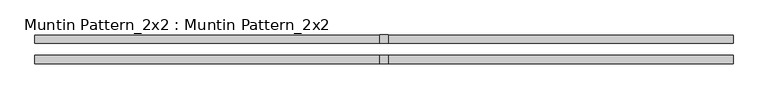
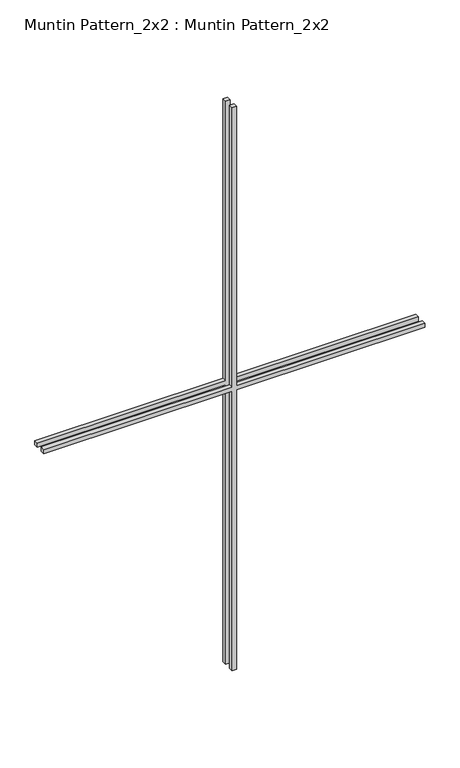
"""IFC4 building model written with IfcOpenShell, lengths in millimetres: proxy geometry, Muntin Pattern_2x2 : Muntin Pattern_2x2."""

from ifc_helpers import new_model, si_unit, frame, origin, place, context, project, spatial, polyline, outline, extrude, source, transform, mapped, element, save


def muntin_pattern_2x2_muntin_pattern_2x2_d03a1f3c(model_context):
    return source(origin(), model_context, "Body", "SweptSolid", [
        extrude(outline(polyline([(850.9, -6.35), (850.9, -541.3375), (838.2, -541.3375), (838.2, -6.35), (0.0, -6.35), (0.0, 6.35), (838.2, 6.35), (838.2, 541.3375), (850.9, 541.3375), (850.9, 6.35), (1689.1, 6.35), (1689.1, -6.35), (850.9, -6.35)])), frame((0.0, -22.225, 0.0), z_axis=(0.0, 1.0, 0.0), x_axis=(0.0, 0.0, 1.0)), (0.0, 0.0, 1.0), 12.7),
        extrude(outline(polyline([(850.9, -6.35), (850.9, -541.3375), (838.2, -541.3375), (838.2, -6.35), (0.0, -6.35), (0.0, 6.35), (838.2, 6.35), (838.2, 541.3375), (850.9, 541.3375), (850.9, 6.35), (1689.1, 6.35), (1689.1, -6.35), (850.9, -6.35)])), frame((0.0, 9.525, 0.0), z_axis=(0.0, 1.0, 0.0), x_axis=(0.0, 0.0, 1.0)), (0.0, 0.0, 1.0), 12.7),
    ])


if __name__ == "__main__":
    model = new_model("IFC4")
    model_context = context("Model", 3, world=origin())
    ifc_project = project(units=[si_unit("LENGTHUNIT", "METRE", prefix="MILLI")], contexts=[model_context])
    site = spatial("IfcSite", under=ifc_project)
    building = spatial("IfcBuilding", under=site)
    placement = place(None, origin())
    muntin_pattern_2x2_muntin_pattern_2x2_shape = muntin_pattern_2x2_muntin_pattern_2x2_d03a1f3c(model_context)
    element("IfcBuildingElementProxy", 1, Name="Muntin Pattern_2x2 : Muntin Pattern_2x2", ObjectType="Muntin Pattern_2x2 : Muntin Pattern_2x2", at=placement, inside=building, context=model_context, shape_type="MappedRepresentation", body=[
        mapped(muntin_pattern_2x2_muntin_pattern_2x2_shape, transform((0.0, 0.0, 0.0), x_axis=(1.0, 0.0, 0.0), y_axis=(0.0, 1.0, 0.0), z_axis=(0.0, 0.0, 1.0))),
    ])
    save(model, "model.ifc")

# Revit data of these elements
# Type "Muntin Pattern_2x2 : Muntin Pattern_2x2"
#   Width [instance default] = 4' - 0"
#   Thickness = 0' - 0 1/2"
#   Height [instance default] = 4' - 0"
#   Distance = 0' - 0 3/4"
#   Interior Material [instance default] = none
#   Exterior Material [instance default] = none
#   Default Elevation = 0
# Element 1 (IfcBuildingElementProxy, "Muntin Pattern_2x2 : Muntin Pattern_2x2")
#   Width = 3' - 6 5/8"
#   Height = 5' - 6 1/2"
#   Interior Material = Wood - Stained
#   Exterior Material = Clad - White
#   Materials on its faces: "Clad - White", "Wood - Stained"
# Materials
#   "Clad - White": class "Wood", colour RGB 242 242 238, transparency 0, Cost = 0
#   "Wood - Stained": class "Wood", colour RGB 224 178 126, transparency 0, Cost = 0
